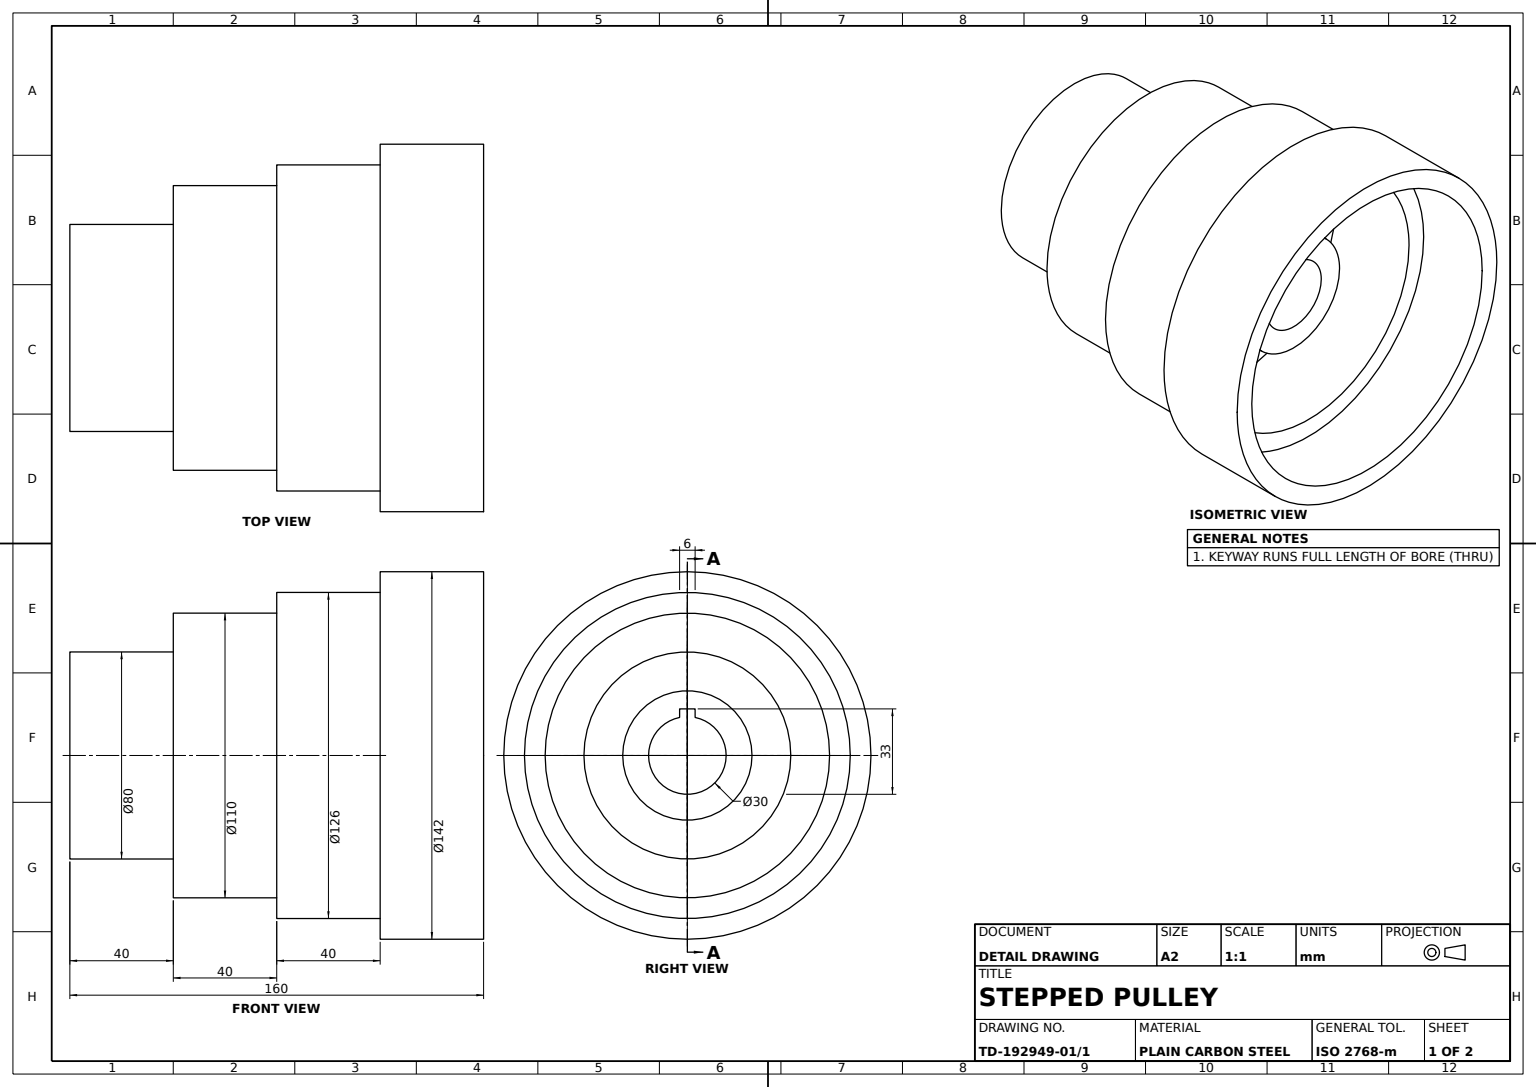
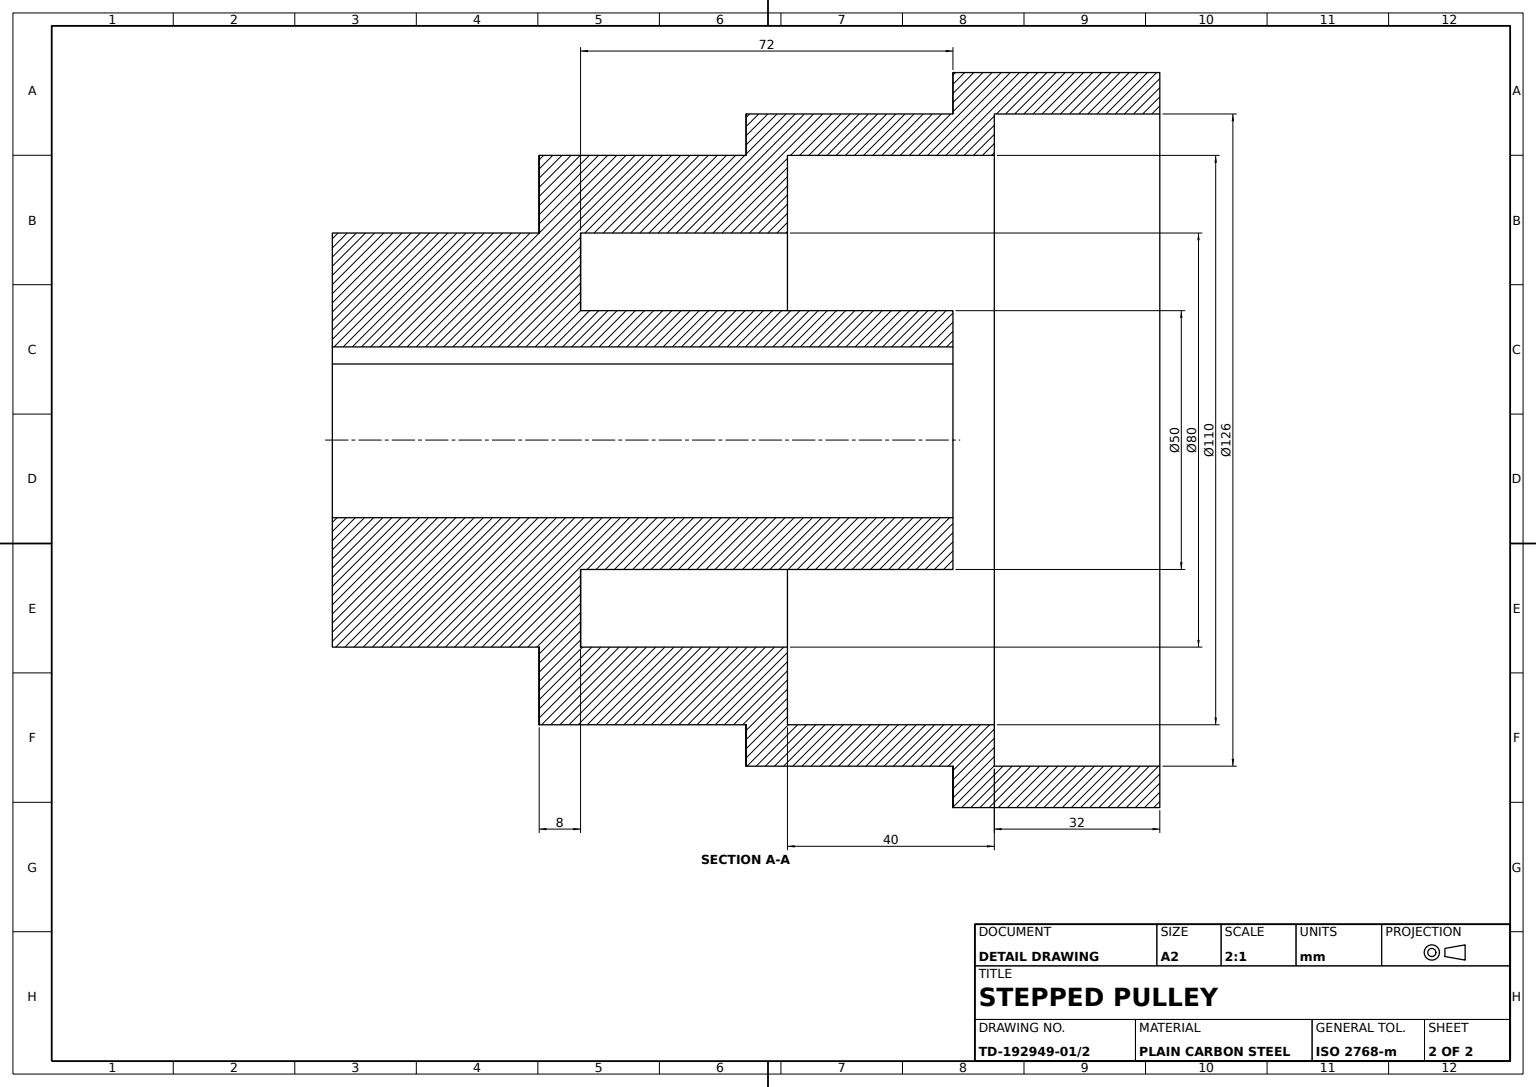
SolidWorks part; units mm, degrees
material "Plain Carbon Steel"
ref_plane "Front Plane" through (0, 0, 0) normal (0, 0, 1) x (1, 0, 0)
ref_plane "Top Plane" through (0, 0, 0) normal (0, 1, 0) x (1, 0, 0)
ref_plane "Right Plane" through (0, 0, 0) normal (1, 0, 0) x (0, 0, -1)
sketch "Pulley Step Profile" plane through (0, 0, 0) normal (0, 0, 1) x (1, 0, 0)
  line L0 (-51.5789, 0) -> (187.6316, 0) construction
  line L1 (0, 77.6316) -> (0, -87.1053) construction
  line L2 (0, 40) -> (0, 15)
  line L4 (0, 40) -> (40, 40)
  line L5 (40, 40) -> (40, 55)
  line L6 (40, 55) -> (80, 55)
  line L7 (80, 55) -> (80, 63)
  line L8 (80, 63) -> (120, 63)
  line L9 (120, 63) -> (120, 71)
  line L10 (120, 71) -> (160, 71)
  line L11 (160, 71) -> (160, 63)
  line L12 (160, 63) -> (128, 63)
  line L13 (128, 63) -> (128, 55)
  line L14 (128, 55) -> (88, 55)
  line L15 (88, 55) -> (88, 40)
  line L16 (88, 40) -> (48, 40)
  line L17 (48, 40) -> (48, 25)
  line L18 (48, 25) -> (120, 25)
  line L19 (120, 25) -> (120, 15)
  line L20 (120, 15) -> (0, 15)
  point P25 (40, 47.5)
  dimension "D1" = 15
  dimension "D2" = 40
  dimension "D3" = 40
  dimension "D4" = 40
  dimension "D5" = 40
  dimension "D6" = 40
  dimension "D7" = 8
  dimension "D8" = 8
  dimension "D9" = 8
  dimension "D10" = 8
  dimension "D11" = 8
  dimension "D12" = 10
  dimension "D13" = 55
  dimension "D14" = 120
revolve "Stepped Pulley Body" add sketch "Pulley Step Profile" angle 360 about L0
sketch "Keyway Profile 6x6" plane through (0, 0, 0) normal (-1, 0, 0) x (0, 0, 1)
  line L1 (-3, 18) -> (3, 18)
  line L2 (-3, 18) -> (-3, 12)
  line L3 (-3, 12) -> (3, 12)
  line L4 (3, 18) -> (3, 12)
  line L5 (-3, 18) -> (3, 12) construction
  line L6 (-3, 12) -> (3, 18) construction
  circle A0 centre (0, 0) radius 15 construction
  point P0 (0, 15)
  dimension "D1" = 6
  dimension "D2" = 6
  dimension "D3" = 3
extrude "Keyway Cut 6x6" cut sketch "Keyway Profile 6x6" against normal blind 211
